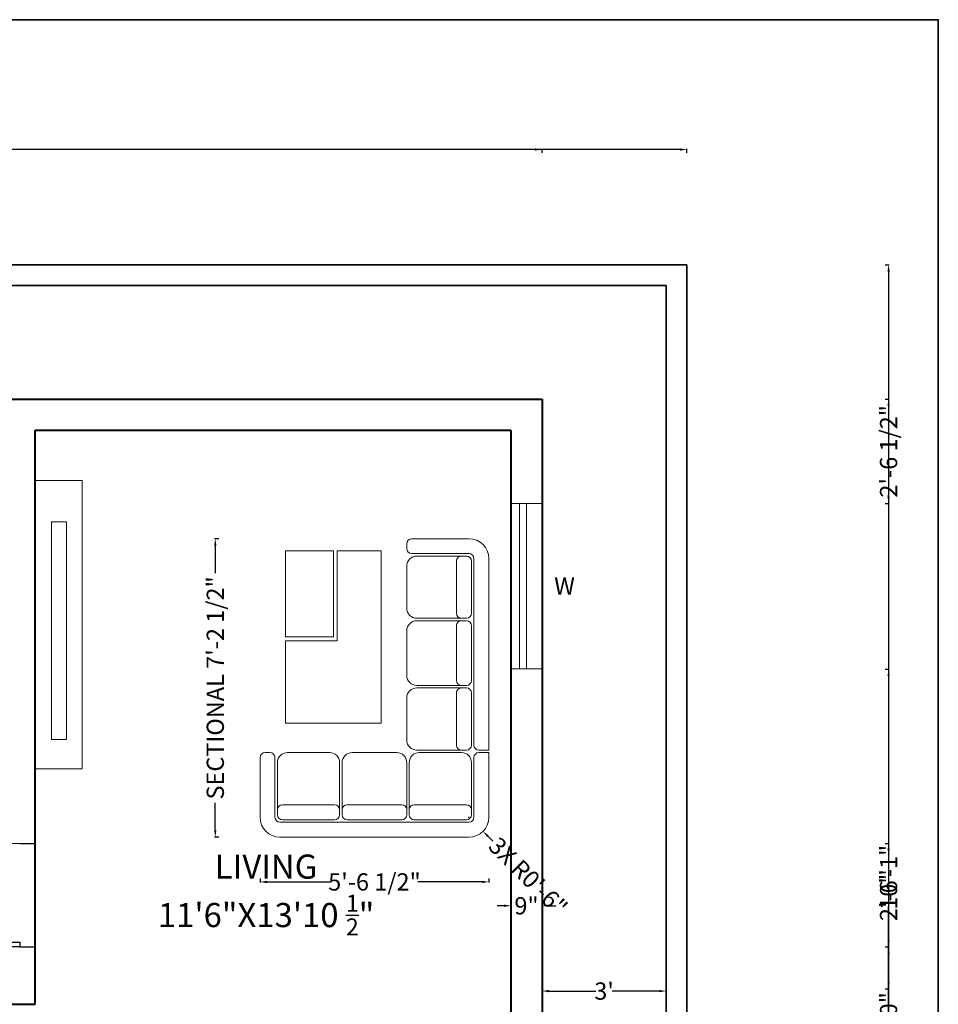
# Model space of a CAD drawing. Units: inches. Extents: x -231 to 349, y -511 to 252.
# Tile 6 of 6: x 82 to 349, y -33 to 252. Entities that reach past the tile are written whole.
import ezdxf

# ---------------------------------------------------------------- set-up
doc = ezdxf.new("R2010")
doc.units = ezdxf.units.IN
doc.header["$MEASUREMENT"] = 0
for name, color, linetype, lineweight in [('A-ANNO-DIMS', 7, 'Continuous', 18), ('A-ANNO-TEXT', 7, 'Continuous', 18), ('A-ANNO-TTLB', 7, 'Continuous', 35), ('A-AREA-IDEN', 7, 'Continuous', 25), ('A-FURN', 8, 'Continuous', 18), ('A-GLAZ', 177, 'Continuous', 20), ('A-WALL', 7, 'Continuous', 40), ('C-PROP', 7, 'Continuous', 35), ('DOOR', 42, 'Continuous', 25)]:
    doc.layers.add(name, color=color, linetype=linetype, lineweight=lineweight)
doc.styles.get("Standard").update_dxf_attribs({"font": 'arial.ttf'})
doc.dimstyles.get("Standard").update_dxf_attribs({"dimtxt": 5, "dimasz": 2, "dimexe": 0.18, "dimexo": 0.0625, "dimgap": 0.09, "dimtad": 0, "dimzin": 0, "dimdsep": 46, "dimlunit": 4, "dimtxsty": 'Standard', "dimcen": 0.09, "dimadec": 0, "dimazin": 0, "dimtfac": 1, "dimtofl": 0, "dimtmove": 0, "dimatfit": 3, "dimfxl": 1, "dimfxlon": 1, "dimtolj": 1, "dimtzin": 0, "dimarcsym": 0})

# ---------------------------------------------------------------- blocks, each defined once
blk = doc.blocks.new('*U2')
for p, q in [((0, 0), (0, -6)), ((40, 0), (40, -6))]:
    blk.add_line(p, q)
blk.add_lwpolyline([(0, 0), (0, 40), (1.75, 40), (1.75, 0)], close=True)
blk.add_arc((0, 0), 40, 0, 90)
blk = doc.blocks.new('A$C2AFA021D')
for p, q in [((0.8, 2.3), (0.2, 2.3)), ((0.85, 2.2), (0.85, 2.25)), ((0, 2.1), (0, 0.2)), ((0.15, 0.2), (0.15, 2.1)), ((0.2, 2.15), (0.8, 2.15)), ((0.225, 2.125), (0.275, 2.125)), ((0.75, 2.125), (0.275, 2.125)), ((0.175, 1.55), (0.175, 2.075)), ((0.325, 2.075), (0.325, 1.55)), ((0.85, 1.6), (0.85, 2.025)), ((0.275, 1.5), (0.225, 1.5)), ((0.275, 1.5), (0.75, 1.5)), ((0.175, 0.875), (0.175, 1.425)), ((0.225, 1.475), (0.275, 1.475)), ((0.75, 1.475), (0.275, 1.475)), ((0.325, 1.425), (0.325, 0.875)), ((0.85, 0.925), (0.85, 1.375)), ((0.275, 0.825), (0.225, 0.825)), ((0.225, 0.8), (0.275, 0.8)), ((0.275, 0.825), (0.75, 0.825)), ((0.75, 0.8), (0.275, 0.8)), ((0.975, 0.825), (1.4, 0.825)), ((1.625, 0.825), (2.075, 0.825)), ((2.3, 0.825), (2.725, 0.825)), ((2.9, 0.825), (2.95, 0.825)), ((0.175, 0.225), (0.175, 0.75)), ((0.325, 0.75), (0.325, 0.225)), ((0.85, 0.275), (0.85, 0.7)), ((0.875, 0.275), (0.875, 0.725)), ((1.5, 0.725), (1.5, 0.275)), ((1.525, 0.275), (1.525, 0.725)), ((2.175, 0.725), (2.175, 0.275)), ((2.2, 0.275), (2.2, 0.725)), ((2.825, 0.725), (2.825, 0.275)), ((2.85, 0.2), (2.85, 0.775)), ((3, 0.775), (3, 0.2)), ((1.45, 0.325), (0.925, 0.325)), ((2.125, 0.325), (1.575, 0.325)), ((2.775, 0.325), (2.25, 0.325)), ((0.875, 0.275), (0.875, 0.225)), ((1.5, 0.225), (1.5, 0.275)), ((1.525, 0.275), (1.525, 0.225)), ((2.175, 0.225), (2.175, 0.275)), ((2.2, 0.275), (2.2, 0.225)), ((2.825, 0.225), (2.825, 0.275)), ((0.8, 0.15), (0.2, 0.15)), ((0.275, 0.175), (0.225, 0.175)), ((0.275, 0.175), (0.75, 0.175)), ((0.85, 0), (0.85, 0.1)), ((0.875, 0.1), (0.875, 0)), ((0.925, 0.175), (1.45, 0.175)), ((0.925, 0.15), (2.8, 0.15)), ((1.575, 0.175), (2.125, 0.175)), ((2.25, 0.175), (2.775, 0.175)), ((0.2, 0), (0.85, 0)), ((2.8, 0), (0.875, 0))]:
    blk.add_line(p, q)
for centre, radius, start, end in [((0.2, 2.1), 0.2, 90, 180), ((0.8, 2.25), 0.05, 0, 90), ((0.8, 2.2), 0.05, 270, 0), ((0.2, 2.1), 0.05, 90, 180), ((0.225, 2.075), 0.05, 90, 180), ((0.275, 2.075), 0.05, 0, 90), ((0.75, 2.025), 0.1, 0, 90), ((0.75, 1.6), 0.1, 270, 0), ((0.225, 1.55), 0.05, 180, 270), ((0.275, 1.55), 0.05, 270, 0), ((0.225, 1.425), 0.05, 90, 180), ((0.275, 1.425), 0.05, 0, 90), ((0.75, 1.375), 0.1, 360, 90), ((0.75, 0.925), 0.1, 270, 0), ((0.225, 0.875), 0.05, 180, 270), ((0.225, 0.75), 0.05, 90, 180), ((0.275, 0.875), 0.05, 270, 0), ((0.275, 0.75), 0.05, 0, 90), ((0.75, 0.7), 0.1, 0, 90), ((0.975, 0.725), 0.1, 90, 180), ((1.4, 0.725), 0.1, 0, 90), ((1.625, 0.725), 0.1, 90, 180), ((2.075, 0.725), 0.1, 0, 90), ((2.3, 0.725), 0.1, 90, 180), ((2.725, 0.725), 0.1, 0, 90), ((2.9, 0.775), 0.05, 90, 180), ((2.95, 0.775), 0.05, 0, 90), ((0.925, 0.275), 0.05, 90, 180), ((1.45, 0.275), 0.05, 360, 90), ((1.575, 0.275), 0.05, 90, 180), ((2.125, 0.275), 0.05, 360, 90), ((2.25, 0.275), 0.05, 90, 180), ((2.775, 0.275), 0.05, 360, 90), ((0.2, 0.2), 0.2, 180, 270), ((0.2, 0.2), 0.05, 180, 270), ((0.225, 0.225), 0.05, 180, 270), ((0.275, 0.225), 0.05, 270, 0), ((0.75, 0.275), 0.1, 270, 0), ((0.925, 0.225), 0.05, 180, 270), ((1.45, 0.225), 0.05, 270, 0), ((1.575, 0.225), 0.05, 180, 270), ((2.125, 0.225), 0.05, 270, 0), ((2.25, 0.225), 0.05, 180, 270), ((2.775, 0.225), 0.05, 270, 0), ((2.8, 0.2), 0.2, 270, 0), ((2.8, 0.2), 0.05, 270, 0), ((0.8, 0.1), 0.05, 0, 90), ((0.925, 0.1), 0.05, 90, 180)]:
    blk.add_arc(centre, radius, start, end)
blk = doc.blocks.new('*D15')
at = {"layer": 'A-ANNO-DIMS', "color": 0, "lineweight": -2, "transparency": 16777216}
for p, q in [((222.92, -4.54), (220.92, -4.54)), ((224.92, -3.95), (224.92, -4.72)), ((233.92, -3.95), (233.92, -4.72)), ((235.92, -4.54), (237.92, -4.54))]:
    blk.add_line(p, q, dxfattribs=at)
at = {"layer": 'A-ANNO-DIMS', "color": 0, "transparency": 16777216}
for points in [[(222.92, -4.2), (222.92, -4.87), (224.92, -4.54)], [(235.92, -4.2), (235.92, -4.87), (233.92, -4.54)]]:
    blk.add_solid(points, dxfattribs=at)
at = {"layer": 'Defpoints', "color": 0, "transparency": 16777216}
for p in [(224.92, -3.88), (233.92, -3.88), (233.92, -4.54)]:
    blk.add_point(p, dxfattribs=at)
at = {"layer": 'A-ANNO-DIMS', "color": 0, "transparency": 16777216, "insert": (229.42, -4.54), "char_height": 5, "attachment_point": 5}
blk.add_mtext('\\A1;9"', dxfattribs=at)
blk = doc.blocks.new('*D20')
at = {"layer": 'A-ANNO-DIMS', "color": 0, "lineweight": -2, "transparency": 16777216}
for p, q in [((233.92, -30.28), (233.92, -29.1)), ((235.92, -29.28), (249.53, -29.28)), ((267.92, -29.28), (254.31, -29.28)), ((269.92, -30.28), (269.92, -29.1))]:
    blk.add_line(p, q, dxfattribs=at)
at = {"layer": 'A-ANNO-DIMS', "color": 0, "transparency": 16777216}
for points in [[(235.92, -28.95), (235.92, -29.62), (233.92, -29.28)], [(267.92, -28.95), (267.92, -29.62), (269.92, -29.28)]]:
    blk.add_solid(points, dxfattribs=at)
at = {"layer": 'Defpoints', "color": 0, "transparency": 16777216}
for p in [(269.92, -29.28), (233.92, -31.56), (269.92, -31.56)]:
    blk.add_point(p, dxfattribs=at)
at = {"layer": 'A-ANNO-DIMS', "color": 0, "transparency": 16777216, "insert": (251.92, -29.28), "char_height": 5, "attachment_point": 5}
blk.add_mtext("\\A1;3'", dxfattribs=at)
blk = doc.blocks.new('WIN-48IN')
for p, q in [((224.92, -56.7), (233.92, -56.7)), ((227.42, -56.7), (227.42, -104.7)), ((229.42, -56.7), (229.42, -104.7)), ((224.92, -104.7), (233.92, -104.7))]:
    blk.add_line(p, q)
blk = doc.blocks.new('*D36')
at = {"layer": 'A-ANNO-DIMS', "color": 0, "lineweight": -2, "transparency": 16777216}
for p, q in [((140.15, 101.92), (138.97, 101.92)), ((139.15, 99.92), (139.15, 91.95)), ((139.15, 17.35), (139.15, 25.32)), ((140.15, 15.35), (138.97, 15.35))]:
    blk.add_line(p, q, dxfattribs=at)
at = {"layer": 'A-ANNO-DIMS', "color": 0, "transparency": 16777216}
for points in [[(138.82, 99.92), (139.48, 99.92), (139.15, 101.92)], [(138.82, 17.35), (139.48, 17.35), (139.15, 15.35)]]:
    blk.add_solid(points, dxfattribs=at)
at = {"layer": 'Defpoints', "color": 0, "transparency": 16777216}
for p in [(139.15, 101.92), (152.13, 101.92), (152.13, 15.35)]:
    blk.add_point(p, dxfattribs=at)
at = {"layer": 'A-ANNO-DIMS', "color": 0, "transparency": 16777216, "insert": (139.15, 58.64), "char_height": 5, "attachment_point": 5, "rotation": 90}
blk.add_mtext('\\A1;SECTIONAL 7\'-2 1/2"', dxfattribs=at)
blk = doc.blocks.new('*D37')
at = {"layer": 'A-ANNO-DIMS', "color": 0, "lineweight": -2, "transparency": 16777216}
for p, q in [((152.13, 3.37), (152.13, 2.19)), ((218.5, 3.37), (218.5, 2.19)), ((154.13, 2.37), (172.75, 2.37)), ((216.5, 2.37), (197.88, 2.37))]:
    blk.add_line(p, q, dxfattribs=at)
at = {"layer": 'A-ANNO-DIMS', "color": 0, "transparency": 16777216}
for points in [[(154.13, 2.7), (154.13, 2.04), (152.13, 2.37)], [(216.5, 2.7), (216.5, 2.04), (218.5, 2.37)]]:
    blk.add_solid(points, dxfattribs=at)
at = {"layer": 'Defpoints', "color": 0, "transparency": 16777216}
for p in [(152.13, 15.35), (218.5, 15.35), (152.13, 2.37)]:
    blk.add_point(p, dxfattribs=at)
at = {"layer": 'A-ANNO-DIMS', "color": 0, "transparency": 16777216, "insert": (185.32, 2.37), "char_height": 5, "attachment_point": 5}
blk.add_mtext('\\A1;5\'-6 1/2"', dxfattribs=at)
blk = doc.blocks.new('*D44')
at = {"layer": 'A-ANNO-DIMS', "color": 0, "lineweight": -2, "transparency": 16777216}
for p, q in [((-156.08, 213.78), (-156.08, 214.96)), ((-154.08, 214.78), (51.24, 214.78)), ((273.92, 214.78), (68.6, 214.78)), ((275.92, 213.78), (275.92, 214.96))]:
    blk.add_line(p, q, dxfattribs=at)
at = {"layer": 'A-ANNO-DIMS', "color": 0, "transparency": 16777216}
for points in [[(-154.08, 215.11), (-154.08, 214.45), (-156.08, 214.78)], [(273.92, 215.11), (273.92, 214.45), (275.92, 214.78)]]:
    blk.add_solid(points, dxfattribs=at)
at = {"layer": 'Defpoints', "color": 0, "transparency": 16777216}
for p in [(275.92, 214.78), (-156.08, 181.38), (275.92, 181.38)]:
    blk.add_point(p, dxfattribs=at)
at = {"layer": 'A-ANNO-DIMS', "color": 0, "transparency": 16777216, "insert": (59.92, 214.78), "char_height": 5, "attachment_point": 5}
blk.add_mtext('\\A1;36\'-0"', dxfattribs=at)
blk = doc.blocks.new('*D45')
at = {"layer": 'A-ANNO-DIMS', "color": 0, "lineweight": -2, "transparency": 16777216}
for p, q in [((333.44, 181.38), (334.62, 181.38)), ((334.44, 179.38), (334.44, -97.84)), ((334.44, -392.62), (334.44, -115.4)), ((333.44, -394.62), (334.62, -394.62))]:
    blk.add_line(p, q, dxfattribs=at)
at = {"layer": 'A-ANNO-DIMS', "color": 0, "transparency": 16777216}
for points in [[(334.11, 179.38), (334.78, 179.38), (334.44, 181.38)], [(334.11, -392.62), (334.78, -392.62), (334.44, -394.62)]]:
    blk.add_solid(points, dxfattribs=at)
at = {"layer": 'Defpoints', "color": 0, "transparency": 16777216}
for p in [(275.92, 181.38), (275.92, -394.62), (334.44, -394.62)]:
    blk.add_point(p, dxfattribs=at)
at = {"layer": 'A-ANNO-DIMS', "color": 0, "transparency": 16777216, "insert": (334.44, -106.62), "char_height": 5, "attachment_point": 5, "rotation": 90}
blk.add_mtext('\\A1;48\'-0"', dxfattribs=at)
blk = doc.blocks.new('*D46')
at = {"layer": 'A-ANNO-DIMS', "color": 0, "lineweight": -2, "transparency": 16777216}
for p, q in [((-117.08, 213.78), (-117.08, 214.96)), ((-115.08, 214.78), (49.7, 214.78)), ((231.92, 214.78), (67.14, 214.78)), ((233.92, 213.78), (233.92, 214.96))]:
    blk.add_line(p, q, dxfattribs=at)
at = {"layer": 'A-ANNO-DIMS', "color": 0, "transparency": 16777216}
for points in [[(-115.08, 215.11), (-115.08, 214.45), (-117.08, 214.78)], [(231.92, 215.11), (231.92, 214.45), (233.92, 214.78)]]:
    blk.add_solid(points, dxfattribs=at)
at = {"layer": 'Defpoints', "color": 0, "transparency": 16777216}
for p in [(233.92, 214.78), (-117.08, 142.38), (233.92, 142.38)]:
    blk.add_point(p, dxfattribs=at)
at = {"layer": 'A-ANNO-DIMS', "color": 0, "transparency": 16777216, "insert": (58.42, 214.78), "char_height": 5, "attachment_point": 5}
blk.add_mtext('\\A1;29\'-3"', dxfattribs=at)
blk = doc.blocks.new('*D54')
at = {"layer": 'A-ANNO-DIMS', "color": 0, "lineweight": -2, "transparency": 16777216}
for p, q in [((333.44, 142.38), (334.62, 142.38)), ((334.44, 140.38), (334.44, 139.86)), ((334.44, 114.12), (334.44, 114.65)), ((333.44, 112.12), (334.62, 112.12))]:
    blk.add_line(p, q, dxfattribs=at)
at = {"layer": 'A-ANNO-DIMS', "color": 0, "transparency": 16777216}
for points in [[(334.11, 140.38), (334.78, 140.38), (334.44, 142.38)], [(334.11, 114.12), (334.78, 114.12), (334.44, 112.12)]]:
    blk.add_solid(points, dxfattribs=at)
at = {"layer": 'Defpoints', "color": 0, "transparency": 16777216}
for p in [(233.92, 142.38), (233.92, 112.12), (334.44, 112.12)]:
    blk.add_point(p, dxfattribs=at)
at = {"layer": 'A-ANNO-DIMS', "color": 0, "transparency": 16777216, "insert": (334.44, 127.25), "char_height": 5, "attachment_point": 5, "rotation": 90}
blk.add_mtext('\\A1;2\'-6 1/2"', dxfattribs=at)
blk = doc.blocks.new('*D55')
at = {"layer": 'A-ANNO-DIMS', "color": 0, "lineweight": -2, "transparency": 16777216}
for p, q in [((333.44, 64.12), (334.62, 64.12)), ((334.44, 62.12), (334.44, 12.15)), ((334.44, -54.7), (334.44, -4.73)), ((333.44, -56.7), (334.62, -56.7))]:
    blk.add_line(p, q, dxfattribs=at)
at = {"layer": 'A-ANNO-DIMS', "color": 0, "transparency": 16777216}
for points in [[(334.11, 62.12), (334.78, 62.12), (334.44, 64.12)], [(334.11, -54.7), (334.78, -54.7), (334.44, -56.7)]]:
    blk.add_solid(points, dxfattribs=at)
at = {"layer": 'Defpoints', "color": 0, "transparency": 16777216}
for p in [(233.92, 64.12), (233.92, -56.7), (334.44, -56.7)]:
    blk.add_point(p, dxfattribs=at)
at = {"layer": 'A-ANNO-DIMS', "color": 0, "transparency": 16777216, "insert": (334.44, 3.71), "char_height": 5, "attachment_point": 5, "rotation": 90}
blk.add_mtext('\\A1;10\'-1"', dxfattribs=at)
blk = doc.blocks.new('*D63')
at = {"layer": 'A-ANNO-DIMS', "color": 0, "lineweight": -2, "transparency": 16777216}
for p, q in [((333.44, 13.54), (334.62, 13.54)), ((334.44, 11.54), (334.44, 5.32)), ((334.44, -14.46), (334.44, -8.24)), ((333.44, -16.46), (334.62, -16.46))]:
    blk.add_line(p, q, dxfattribs=at)
at = {"layer": 'A-ANNO-DIMS', "color": 0, "transparency": 16777216}
for points in [[(334.11, 11.54), (334.78, 11.54), (334.44, 13.54)], [(334.11, -14.46), (334.78, -14.46), (334.44, -16.46)]]:
    blk.add_solid(points, dxfattribs=at)
at = {"layer": 'Defpoints', "color": 0, "transparency": 16777216}
for p in [(86.92, 13.54), (86.92, -16.46), (334.44, -16.46)]:
    blk.add_point(p, dxfattribs=at)
at = {"layer": 'A-ANNO-DIMS', "color": 0, "transparency": 16777216, "insert": (334.44, -1.46), "char_height": 5, "attachment_point": 5, "rotation": 90}
blk.add_mtext('\\A1;2\'-6"', dxfattribs=at)
blk = doc.blocks.new('*D64')
at = {"layer": 'A-ANNO-DIMS', "color": 0, "lineweight": -2, "transparency": 16777216}
for p, q in [((333.44, -16.46), (334.62, -16.46)), ((334.44, -18.46), (334.44, -26.62)), ((333.44, -28.62), (334.62, -28.62)), ((334.44, -28.62), (334.44, -30.62))]:
    blk.add_line(p, q, dxfattribs=at)
at = {"layer": 'A-ANNO-DIMS', "color": 0, "transparency": 16777216}
for points in [[(334.11, -18.46), (334.78, -18.46), (334.44, -16.46)], [(334.11, -26.62), (334.78, -26.62), (334.44, -28.62)]]:
    blk.add_solid(points, dxfattribs=at)
at = {"layer": 'Defpoints', "color": 0, "transparency": 16777216}
for p in [(82.42, -16.46), (82.42, -28.62), (334.44, -28.62)]:
    blk.add_point(p, dxfattribs=at)
at = {"layer": 'A-ANNO-DIMS', "color": 0, "transparency": 16777216, "insert": (334.44, -37.12), "char_height": 5, "attachment_point": 5, "rotation": 90}
blk.add_mtext('\\A1;1\'-0"', dxfattribs=at)
blk = doc.blocks.new('*D69')
at = {"layer": 'A-ANNO-DIMS', "color": 0, "lineweight": -2, "transparency": 16777216}
for p, q in [((212.64, 21.13), (212.82, 21.13)), ((212.73, 21.04), (212.73, 21.22)), ((219.64, 14.22), (218.22, 15.63))]:
    blk.add_line(p, q, dxfattribs=at)
at = {"layer": 'A-ANNO-DIMS', "color": 0, "transparency": 16777216}
blk.add_solid([(218.46, 15.87), (217.99, 15.4), (216.81, 17.05)], dxfattribs=at)
at = {"layer": 'Defpoints', "color": 0, "transparency": 16777216}
for p in [(212.73, 21.13), (216.81, 17.05)]:
    blk.add_point(p, dxfattribs=at)
at = {"layer": 'A-ANNO-DIMS', "color": 0, "transparency": 16777216, "insert": (229.89, 3.97), "char_height": 5, "attachment_point": 5, "rotation": 315.0024}
blk.add_mtext('\\A1;3X R0\'-6"', dxfattribs=at)

msp = doc.modelspace()

# ---------------------------------------------------------------- linework, layer by layer
at = {"layer": 'A-ANNO-TTLB'}
msp.add_lwpolyline([(-231.158, 252.428), (348.864, 252.428), (348.864, -511.312), (-231.158, -511.312)], close=True, dxfattribs=at)
at = {"layer": 'A-FURN'}
for p, q in [((86.92, 118.777), (100.575, 118.777)), ((100.575, 118.777), (100.575, 35.126)), ((174.54, 98.426), (174.54, 72.293)), ((174.54, 72.293), (159.513, 72.293)), ((100.575, 35.126), (86.92, 35.126))]:
    msp.add_line(p, q, dxfattribs=at)
for points in [[(91.653, 106.826), (96.016, 106.826), (96.016, 43.714), (91.653, 43.714)], [(159.513, 98.426), (173.411, 98.426), (173.411, 73.439), (159.513, 73.439)]]:
    msp.add_lwpolyline(points, close=True, dxfattribs=at)
msp.add_lwpolyline([(174.54, 98.426), (187.31, 98.426), (187.31, 48.452), (159.513, 48.452), (159.513, 72.293)], dxfattribs=at)
at = {"layer": 'A-WALL'}
for p, q in [((-117.08, 142.38), (233.92, 142.38)), ((233.92, 142.38), (233.92, -186.12)), ((86.92, 133.38), (224.92, 133.38)), ((86.92, -33.12), (86.92, 133.38)), ((224.92, 133.38), (224.92, -177.12)), ((23.92, -33.12), (86.92, -33.12))]:
    msp.add_line(p, q, dxfattribs=at)
at = {"layer": 'C-PROP'}
for p, q in [((-156.08, 181.38), (275.92, 181.38)), ((275.92, 181.38), (275.92, -394.62)), ((-150.08, 175.38), (269.92, 175.38)), ((269.92, 175.38), (269.92, -376.62))]:
    msp.add_line(p, q, dxfattribs=at)

# ---------------------------------------------------------------- block references
at = {"layer": 'A-FURN', "xscale": 28.85440272944384, "yscale": 28.85440272944384, "zscale": 28.85440272944384, "rotation": 90}
msp.add_blockref('A$C2AFA021D', (218.498, 15.355), dxfattribs=at)
at = {"layer": 'A-GLAZ'}
msp.add_blockref('WIN-48IN', (0, 168.827), dxfattribs=at)
at = {"layer": 'DOOR', "xscale": 0.75, "yscale": 0.75, "zscale": 0.75, "rotation": 90.00000000000003}
msp.add_blockref('*U2', (82.42, -16.457), dxfattribs=at)

# ---------------------------------------------------------------- texts
at = {"layer": 'A-ANNO-TEXT', "insert": (237.455, 90.664), "char_height": 5, "attachment_point": 1}
msp.add_mtext_dynamic_manual_height_columns('\\A1;W', width=7.82759, gutter_width=1, heights=[0], dxfattribs=at)
at = {"layer": 'A-AREA-IDEN', "insert": (102.562, 10.309), "char_height": 7, "attachment_point": 1}
msp.add_mtext_dynamic_manual_height_columns('\\A1;\\pxqc;LIVING\\P11\'6"X13\'10 {\\H0.7x;\\S1/2;}"', width=102.65834, gutter_width=1, heights=[0], dxfattribs=at)

# ---------------------------------------------------------------- dimensions: what is measured, and where the dimension line sits
at = {"layer": 'A-ANNO-DIMS'}
for base, p1, p2, override, picture, middle in [((275.92, 214.78), (-156.08, 181.38), (275.92, 181.38), {"dimdec": 1, "dimlfac": 1, "dimrnd": 0, "dimzin": 1, "dimdsep": 46, "dimlunit": 4, "dimfrac": 2}, '*D44', (59.92, 214.78)), ((233.92, 214.78), (-117.08, 142.38), (233.92, 142.38), {"dimdec": 1, "dimlfac": 1, "dimrnd": 0, "dimzin": 1, "dimdsep": 46, "dimlunit": 4, "dimfrac": 2}, '*D46', (58.42, 214.78)), ((233.92, -4.536), (224.92, -3.884), (233.92, -3.884), {"dimclrd": 0, "dimclre": 0, "dimclrt": 0}, '*D15', (229.42, -4.536)), ((269.92, -29.284), (233.92, -31.557), (269.92, -31.557), {"dimclrd": 0, "dimclre": 0, "dimclrt": 0}, '*D20', (251.92, -29.284))]:
    dim = msp.add_linear_dim(base=base, p1=p1, p2=p2, dimstyle='Standard', override=override, dxfattribs=at)
    dim.commit()
    dim.dimension.update_dxf_attribs({"geometry": picture, "text_midpoint": middle})
for base, p1, p2, angle, picture, middle in [((334.442, -394.62), (275.92, 181.38), (275.92, -394.62), 90, '*D45', (334.442, -106.62)), ((334.442, 112.123), (233.92, 142.38), (233.92, 112.123), 90, '*D54', (334.442, 127.252)), ((334.442, -56.704), (233.92, 64.123), (233.92, -56.704), 90, '*D55', (334.442, 3.71)), ((152.133, 2.37), (218.498, 15.355), (152.133, 15.355), 180, '*D37', (185.315, 2.37)), ((334.442, -16.457), (86.92, 13.543), (86.92, -16.457), 90, '*D63', (334.442, -1.457)), ((334.442, -28.62), (82.42, -16.457), (82.42, -28.62), 90, '*D64', (334.442, -37.121))]:
    dim = msp.add_linear_dim(base=base, p1=p1, p2=p2, angle=angle, dimstyle='Standard', override={"dimdec": 1, "dimlfac": 1, "dimrnd": 0, "dimzin": 1, "dimdsep": 46, "dimlunit": 4, "dimfrac": 2}, dxfattribs=at)
    dim.commit()
    dim.dimension.update_dxf_attribs({"geometry": picture, "text_midpoint": middle})
dim = msp.add_linear_dim(base=(139.148, 101.918), p1=(152.133, 15.355), p2=(152.133, 101.918), angle=90, text='SECTIONAL <>', dimstyle='Standard', override={"dimdec": 1, "dimlfac": 1, "dimrnd": 0, "dimzin": 1, "dimdsep": 46, "dimlunit": 4, "dimfrac": 2}, dxfattribs=at)
dim.commit()
dim.dimension.update_dxf_attribs({"geometry": '*D36', "text_midpoint": (139.148, 58.636)})
dim = msp.add_radius_dim(center=(212.727, 21.126), mpoint=(216.808, 17.045), text='3X <>', dimstyle='Standard', override={"dimdec": 1, "dimlfac": 1, "dimrnd": 0, "dimzin": 1, "dimdsep": 46, "dimlunit": 4, "dimfrac": 2}, dxfattribs=at)
dim.commit()
dim.dimension.update_dxf_attribs({"geometry": '*D69', "text_midpoint": (229.889, 3.965)})

doc.saveas('drawing.dxf')
